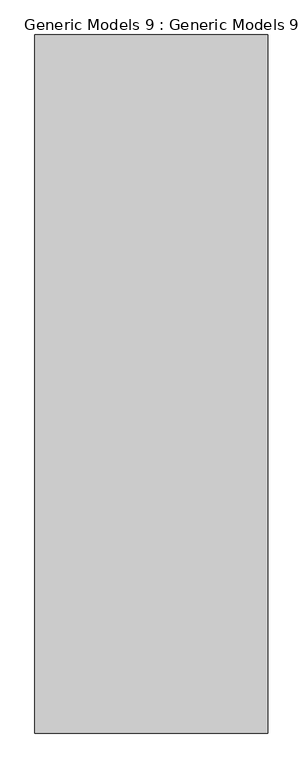
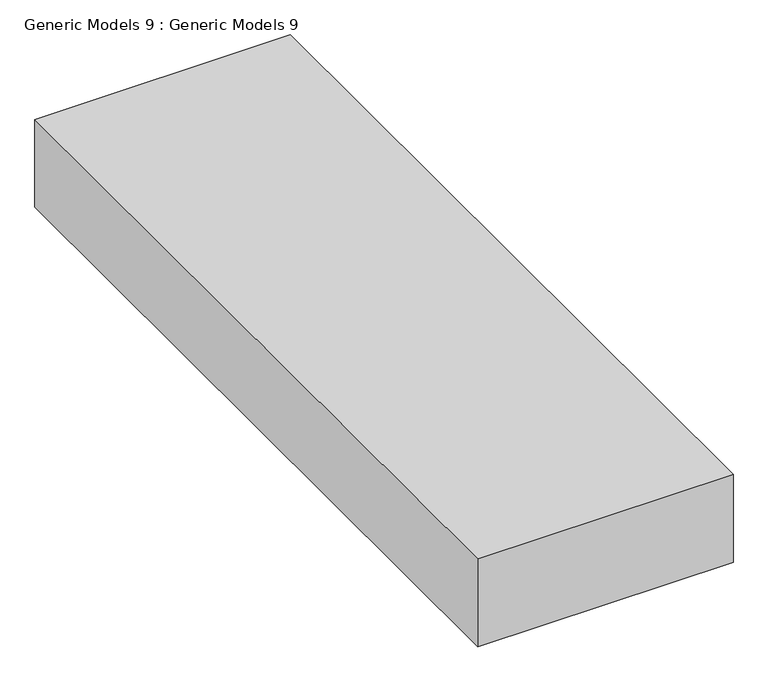
"""IFC4 building model written with IfcOpenShell, lengths in millimetres: proxy geometry, Generic Models 9 : Generic Models 9."""

from ifc_helpers import new_model, si_unit, frame, origin, place, context, project, spatial, polyline, outline, extrude, source, transform, mapped, element, save


def generic_models_9_generic_models_9_222cebfa(model_context):
    return source(origin(), model_context, "Body", "SweptSolid", [
        extrude(outline(polyline([(-5312.6120831, -1.3292064), (-5871.4120831, -1.3292064), (-5871.4120831, 1675.0707936), (-5312.6120831, 1675.0707936), (-5312.6120831, -1.3292064)])), frame((0.0, 0.0, 5376.6144653), z_axis=(0.0, 0.0, 1.0), x_axis=(1.0, 0.0, 0.0)), (0.0, 0.0, 1.0), 203.2),
    ])


if __name__ == "__main__":
    model = new_model("IFC4")
    model_context = context("Model", 3, world=origin())
    ifc_project = project(units=[si_unit("LENGTHUNIT", "METRE", prefix="MILLI")], contexts=[model_context])
    site = spatial("IfcSite", under=ifc_project)
    building = spatial("IfcBuilding", under=site)
    placement = place(None, origin())
    generic_models_9_generic_models_9_shape = generic_models_9_generic_models_9_222cebfa(model_context)
    element("IfcBuildingElementProxy", 1, Name="Generic Models 9 : Generic Models 9", ObjectType="Generic Models 9 : Generic Models 9", at=placement, inside=building, context=model_context, shape_type="MappedRepresentation", body=[
        mapped(generic_models_9_generic_models_9_shape, transform((0.0, 0.0, 0.0), x_axis=(1.0, 0.0, 0.0), y_axis=(0.0, 1.0, 0.0), z_axis=(0.0, 0.0, 1.0))),
    ])
    save(model, "model.ifc")
